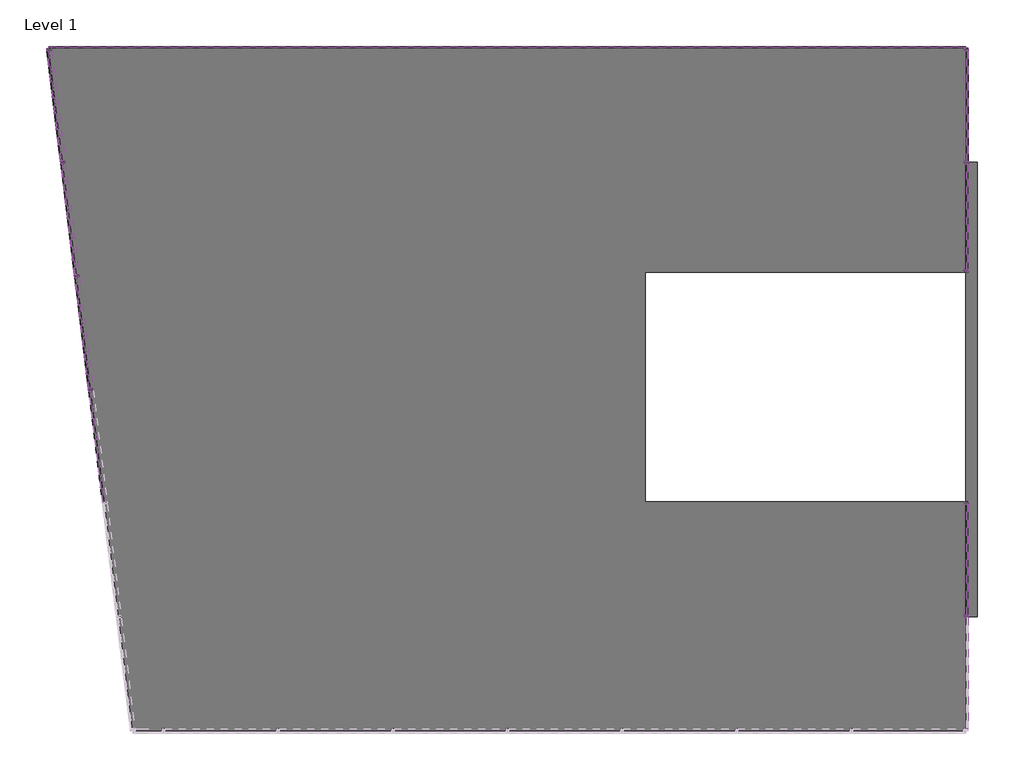
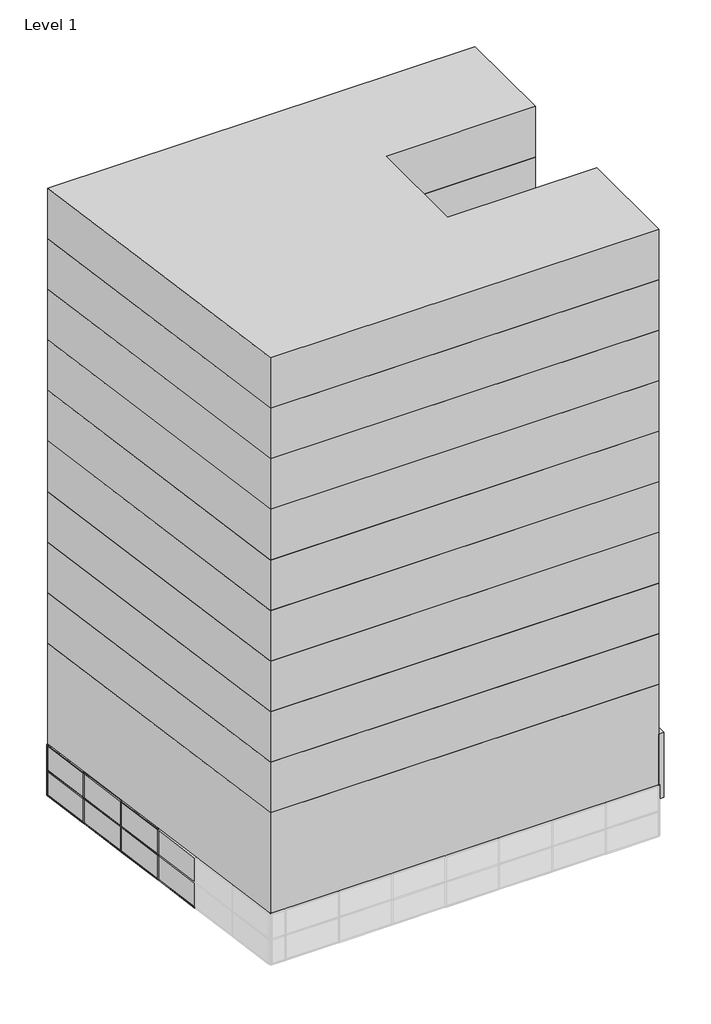
# One storey, part 2 of 2: 38 members, 30 plates, 2 proxies.
"""IFC4 building model written with IfcOpenShell, lengths in millimetres."""

from ifc_helpers import new_model, si_unit, frame, origin, origin_with_axes, place, context, project, spatial, polyline, outline, extrude, transform, mapped, element, save
from components import generic_models_1_generic_models_1_98a022ed, member_71c27fd2, member_19d0a4ec, member_8cef0660, member_db480205, member_82905deb, member_4491d118, member_1b94d493, member_46bdb8c2, system_panel_glazed_1e57f9bb, system_panel_glazed_37f15d2e, system_panel_glazed_3620f98e, system_panel_glazed_e46d4b42, system_panel_glazed_2a6c68b7, system_panel_glazed_7fb1fc2b, system_panel_glazed_d483336f

model = new_model("IFC4")

# Units and contexts
model_context = context("Model", 3, world=origin())
ifc_project = project(units=[si_unit("LENGTHUNIT", "METRE", prefix="MILLI")], contexts=[model_context])

# Site, building, storey
site = spatial("IfcSite", under=ifc_project)
building = spatial("IfcBuilding", under=site)
storey = spatial("IfcBuildingStorey", under=building, Name="Level 1", Elevation=0.0)

# Proxies
placement = place(None, origin())
generic_models_1_generic_models_1_shape = generic_models_1_generic_models_1_98a022ed(model_context)
element("IfcBuildingElementProxy", 1, Name="Generic Models 1 : Generic Models 1", ObjectType="Generic Models 1 : Generic Models 1", at=placement, inside=storey, context=model_context, shape_type="MappedRepresentation", body=[
    mapped(generic_models_1_generic_models_1_shape, transform((0.0, 0.0, 0.0), x_axis=(1.0, 0.0, 0.0), y_axis=(0.0, 1.0, 0.0), z_axis=(0.0, 0.0, 1.0))),
])
element("IfcBuildingElementProxy", 2, Name="Mass 1 : Mass 1", ObjectType="Mass 1 : Mass 1", at=placement, inside=storey, context=model_context, shape_type="SweptSolid", body=[
    extrude(outline(polyline([(13902.5156363, 11172.5476508), (13902.5156363, 5212.8636295), (5368.1156363, 5212.8636295), (5368.1156363, -883.1363705), (13902.5156363, -883.1363705), (13902.5156363, -6979.1363705), (-8252.7378115, -6979.1363705), (-10481.4843637, 11172.5476508), (13902.5156363, 11172.5476508)])), origin_with_axes(), (0.0, 0.0, 1.0), 9144.0),
    extrude(outline(polyline([(13902.5156363, 11172.5476508), (13902.5156363, 5212.8636295), (5368.1156363, 5212.8636295), (5368.1156363, -883.1363705), (13902.5156363, -883.1363705), (13902.5156363, -6979.1363705), (-8252.7378115, -6979.1363705), (-10481.4843637, 11172.5476508), (13902.5156363, 11172.5476508)])), origin_with_axes(), (0.0, 0.0, 1.0), 9144.0),
    extrude(outline(polyline([(13902.5156363, 11172.5476508), (13902.5156363, 5212.8636295), (5368.1156363, 5212.8636295), (5368.1156363, -883.1363705), (13902.5156363, -883.1363705), (13902.5156363, -6979.1363705), (-8252.7378115, -6979.1363705), (-10481.4843637, 11172.5476508), (13902.5156363, 11172.5476508)])), frame((0.0, 0.0, 3048.0), z_axis=(0.0, 0.0, 1.0), x_axis=(1.0, 0.0, 0.0)), (0.0, 0.0, 1.0), 9144.0),
    extrude(outline(polyline([(13902.5156363, 11172.5476508), (13902.5156363, 5212.8636295), (5368.1156363, 5212.8636295), (5368.1156363, -883.1363705), (13902.5156363, -883.1363705), (13902.5156363, -6979.1363705), (-8252.7378115, -6979.1363705), (-10481.4843637, 11172.5476508), (13902.5156363, 11172.5476508)])), frame((0.0, 0.0, 6096.0), z_axis=(0.0, 0.0, 1.0), x_axis=(1.0, 0.0, 0.0)), (0.0, 0.0, 1.0), 9144.0),
    extrude(outline(polyline([(13902.5156363, 11172.5476508), (13902.5156363, 5212.8636295), (5368.1156363, 5212.8636295), (5368.1156363, -883.1363705), (13902.5156363, -883.1363705), (13902.5156363, -6979.1363705), (-8252.7378115, -6979.1363705), (-10481.4843637, 11172.5476508), (13902.5156363, 11172.5476508)])), frame((0.0, 0.0, 9144.0), z_axis=(0.0, 0.0, 1.0), x_axis=(1.0, 0.0, 0.0)), (0.0, 0.0, 1.0), 9144.0),
    extrude(outline(polyline([(13902.5156363, 11172.5476508), (13902.5156363, 5212.8636295), (5368.1156363, 5212.8636295), (5368.1156363, -883.1363705), (13902.5156363, -883.1363705), (13902.5156363, -6979.1363705), (-8252.7378115, -6979.1363705), (-10481.4843637, 11172.5476508), (13902.5156363, 11172.5476508)])), frame((0.0, 0.0, 12192.0), z_axis=(0.0, 0.0, 1.0), x_axis=(1.0, 0.0, 0.0)), (0.0, 0.0, 1.0), 9144.0),
    extrude(outline(polyline([(13902.5156363, 11172.5476508), (13902.5156363, 5212.8636295), (5368.1156363, 5212.8636295), (5368.1156363, -883.1363705), (13902.5156363, -883.1363705), (13902.5156363, -6979.1363705), (-8252.7378115, -6979.1363705), (-10481.4843637, 11172.5476508), (13902.5156363, 11172.5476508)])), frame((0.0, 0.0, 15240.0), z_axis=(0.0, 0.0, 1.0), x_axis=(1.0, 0.0, 0.0)), (0.0, 0.0, 1.0), 9144.0),
    extrude(outline(polyline([(13902.5156363, 11172.5476508), (13902.5156363, 5212.8636295), (5368.1156363, 5212.8636295), (5368.1156363, -883.1363705), (13902.5156363, -883.1363705), (13902.5156363, -6979.1363705), (-8252.7378115, -6979.1363705), (-10481.4843637, 11172.5476508), (13902.5156363, 11172.5476508)])), frame((0.0, 0.0, 18288.0), z_axis=(0.0, 0.0, 1.0), x_axis=(1.0, 0.0, 0.0)), (0.0, 0.0, 1.0), 9144.0),
    extrude(outline(polyline([(13902.5156363, 11172.5476508), (13902.5156363, 5212.8636295), (5368.1156363, 5212.8636295), (5368.1156363, -883.1363705), (13902.5156363, -883.1363705), (13902.5156363, -6979.1363705), (-8252.7378115, -6979.1363705), (-10481.4843637, 11172.5476508), (13902.5156363, 11172.5476508)])), frame((0.0, 0.0, 21336.0), z_axis=(0.0, 0.0, 1.0), x_axis=(1.0, 0.0, 0.0)), (0.0, 0.0, 1.0), 9144.0),
    extrude(outline(polyline([(13902.5156363, 11172.5476508), (13902.5156363, 5212.8636295), (5368.1156363, 5212.8636295), (5368.1156363, -883.1363705), (13902.5156363, -883.1363705), (13902.5156363, -6979.1363705), (-8252.7378115, -6979.1363705), (-10481.4843637, 11172.5476508), (13902.5156363, 11172.5476508)])), frame((0.0, 0.0, 24384.0), z_axis=(0.0, 0.0, 1.0), x_axis=(1.0, 0.0, 0.0)), (0.0, 0.0, 1.0), 9144.0),
    extrude(outline(polyline([(13902.5156363, 11172.5476508), (13902.5156363, 5212.8636295), (5368.1156363, 5212.8636295), (5368.1156363, -883.1363705), (13902.5156363, -883.1363705), (13902.5156363, -6979.1363705), (-8252.7378115, -6979.1363705), (-10481.4843637, 11172.5476508), (13902.5156363, 11172.5476508)])), frame((0.0, 0.0, 27432.0), z_axis=(0.0, 0.0, 1.0), x_axis=(1.0, 0.0, 0.0)), (0.0, 0.0, 1.0), 9144.0),
])

# Members
member_shape = member_71c27fd2(model_context)
element("IfcMember", 3, ObjectType="Rectangular Mullion : 2.5\" x 5\" rectangular", at=placement, inside=storey, context=model_context, shape_type="MappedRepresentation", body=[
    mapped(member_shape, transform((-10473.7456604, 11109.5209701, 0.0), x_axis=(0.0, 0.0, -1.0), y_axis=(-0.9925461516413222, -0.12186934340514595, 0.0), z_axis=(-0.12186934340514594, 0.9925461516413221, 0.0))),
])
element("IfcMember", 4, ObjectType="Rectangular Mullion : 2.5\" x 5\" rectangular", at=placement, inside=storey, context=model_context, shape_type="MappedRepresentation", body=[
    mapped(member_shape, transform((13902.5156363, 8156.2976505, 0.0), x_axis=(0.0, 0.0, -1.0), y_axis=(1.0, 0.0, 0.0), z_axis=(0.0, -1.0, 0.0))),
])
element("IfcMember", 5, ObjectType="Rectangular Mullion : 2.5\" x 5\" rectangular", at=placement, inside=storey, context=model_context, shape_type="MappedRepresentation", body=[
    mapped(member_shape, transform((13902.5156363, -3899.3863708, 0.0), x_axis=(0.0, 0.0, -1.0), y_axis=(1.0, 0.0, 0.0), z_axis=(0.0, -1.0, 0.0))),
])
member_2_shape = member_19d0a4ec(model_context)
element("IfcMember", 6, ObjectType="Rectangular Mullion : 2.5\" x 5\" rectangular", at=placement, inside=storey, context=model_context, shape_type="MappedRepresentation", body=[
    mapped(member_2_shape, transform((-10113.8959567, 8178.7803212, 1524.0), x_axis=(0.0, 0.0, 1.0), y_axis=(-0.9925461516413222, -0.12186934340514595, 0.0), z_axis=(0.12186934340514594, -0.9925461516413221, 0.0))),
])
element("IfcMember", 7, ObjectType="Rectangular Mullion : 2.5\" x 5\" rectangular", at=placement, inside=storey, context=model_context, shape_type="MappedRepresentation", body=[
    mapped(member_2_shape, transform((-10113.8959567, 8178.7803212, 3048.0), x_axis=(0.0, 0.0, 1.0), y_axis=(-0.9925461516413222, -0.12186934340514595, 0.0), z_axis=(0.12186934340514594, -0.9925461516413221, 0.0))),
])
element("IfcMember", 8, ObjectType="Rectangular Mullion : 2.5\" x 5\" rectangular", at=placement, inside=storey, context=model_context, shape_type="MappedRepresentation", body=[
    mapped(member_2_shape, transform((13902.5156363, 11109.0476508, 1524.0), x_axis=(0.0, 0.0, 1.0), y_axis=(1.0, 0.0, 0.0), z_axis=(0.0, 1.0, 0.0))),
])
element("IfcMember", 9, ObjectType="Rectangular Mullion : 2.5\" x 5\" rectangular", at=placement, inside=storey, context=model_context, shape_type="MappedRepresentation", body=[
    mapped(member_2_shape, transform((13902.5156363, 11109.0476508, 3048.0), x_axis=(0.0, 0.0, 1.0), y_axis=(1.0, 0.0, 0.0), z_axis=(0.0, 1.0, 0.0))),
])
element("IfcMember", 10, ObjectType="Rectangular Mullion : 2.5\" x 5\" rectangular", at=placement, inside=storey, context=model_context, shape_type="MappedRepresentation", body=[
    mapped(member_2_shape, transform((13902.5156363, -946.6363705, 1524.0), x_axis=(0.0, 0.0, 1.0), y_axis=(1.0, 0.0, 0.0), z_axis=(0.0, 1.0, 0.0))),
])
element("IfcMember", 11, ObjectType="Rectangular Mullion : 2.5\" x 5\" rectangular", at=placement, inside=storey, context=model_context, shape_type="MappedRepresentation", body=[
    mapped(member_2_shape, transform((13902.5156363, -946.6363705, 3048.0), x_axis=(0.0, 0.0, 1.0), y_axis=(1.0, 0.0, 0.0), z_axis=(0.0, 1.0, 0.0))),
])
element("IfcMember", 12, ObjectType="Rectangular Mullion : 2.5\" x 5\" rectangular", at=placement, inside=storey, context=model_context, shape_type="MappedRepresentation", body=[
    mapped(member_2_shape, transform((13902.5156363, -3962.8863708, 3048.0), x_axis=(0.0, 0.0, 1.0), y_axis=(1.0, 0.0, 0.0), z_axis=(0.0, 1.0, 0.0))),
])
member_3_shape = member_8cef0660(model_context)
element("IfcMember", 13, ObjectType="Rectangular Mullion : 2.5\" x 5\" rectangular", at=placement, inside=storey, context=model_context, shape_type="MappedRepresentation", body=[
    mapped(member_3_shape, transform((-9370.9804393, 2128.2189808, 1524.0), x_axis=(0.0, 0.0, 1.0), y_axis=(-0.9925461516413222, -0.12186934340514596, 0.0), z_axis=(0.12186934340514596, -0.9925461516413222, 0.0))),
])
element("IfcMember", 14, ObjectType="Rectangular Mullion : 2.5\" x 5\" rectangular", at=placement, inside=storey, context=model_context, shape_type="MappedRepresentation", body=[
    mapped(member_3_shape, transform((-9742.438198, 5153.499651, 1524.0), x_axis=(0.0, 0.0, 1.0), y_axis=(-0.9925461516413222, -0.12186934340514596, 0.0), z_axis=(0.12186934340514596, -0.9925461516413222, 0.0))),
])
element("IfcMember", 15, ObjectType="Rectangular Mullion : 2.5\" x 5\" rectangular", at=placement, inside=storey, context=model_context, shape_type="MappedRepresentation", body=[
    mapped(member_3_shape, transform((-9370.9804393, 2128.2189808, 3048.0), x_axis=(0.0, 0.0, 1.0), y_axis=(-0.9925461516413223, -0.12186934340514563, 0.0), z_axis=(0.12186934340514562, -0.9925461516413222, 0.0))),
])
element("IfcMember", 16, ObjectType="Rectangular Mullion : 2.5\" x 5\" rectangular", at=placement, inside=storey, context=model_context, shape_type="MappedRepresentation", body=[
    mapped(member_3_shape, transform((-9742.438198, 5153.499651, 3048.0), x_axis=(0.0, 0.0, 1.0), y_axis=(-0.9925461516413222, -0.12186934340514596, 0.0), z_axis=(0.12186934340514596, -0.9925461516413222, 0.0))),
])
member_4_shape = member_db480205(model_context)
element("IfcMember", 17, ObjectType="Rectangular Mullion : 2.5\" x 5\" rectangular", at=placement, inside=storey, context=model_context, shape_type="MappedRepresentation", body=[
    mapped(member_4_shape, transform((-9363.241736, 2065.1923001, 0.0), x_axis=(0.0, 0.0, -1.0), y_axis=(-0.9925461516413222, -0.12186934340514566, 0.0), z_axis=(-0.12186934340514566, 0.9925461516413222, 0.0))),
])
element("IfcMember", 18, ObjectType="Rectangular Mullion : 2.5\" x 5\" rectangular", at=placement, inside=storey, context=model_context, shape_type="MappedRepresentation", body=[
    mapped(member_4_shape, transform((-9734.6994947, 5090.4729703, 0.0), x_axis=(0.0, 0.0, -1.0), y_axis=(-0.9925461516413222, -0.12186934340514596, 0.0), z_axis=(-0.12186934340514596, 0.9925461516413222, 0.0))),
])
element("IfcMember", 19, ObjectType="Rectangular Mullion : 2.5\" x 5\" rectangular", at=placement, inside=storey, context=model_context, shape_type="MappedRepresentation", body=[
    mapped(member_4_shape, transform((-10106.1572534, 8115.7536405, 0.0), x_axis=(0.0, 0.0, -1.0), y_axis=(-0.9925461516413222, -0.12186934340514596, 0.0), z_axis=(-0.12186934340514596, 0.9925461516413222, 0.0))),
])
member_5_shape = member_82905deb(model_context)
element("IfcMember", 20, ObjectType="Rectangular Mullion : 2.5\" x 5\" rectangular", at=placement, inside=storey, context=model_context, shape_type="MappedRepresentation", body=[
    mapped(member_5_shape, transform((-9367.1110876, 2096.7056405, 1524.0), x_axis=(-0.12186934340514591, 0.9925461516413222, 0.0), y_axis=(-0.9925461516413222, -0.12186934340514591, 0.0), z_axis=(0.0, 0.0, 1.0))),
])
element("IfcMember", 21, ObjectType="Rectangular Mullion : 2.5\" x 5\" rectangular", at=placement, inside=storey, context=model_context, shape_type="MappedRepresentation", body=[
    mapped(member_5_shape, transform((-9738.5688463, 5121.9863107, 1524.0), x_axis=(-0.12186934340514591, 0.9925461516413222, 0.0), y_axis=(-0.9925461516413222, -0.12186934340514591, 0.0), z_axis=(0.0, 0.0, 1.0))),
])
element("IfcMember", 22, ObjectType="Rectangular Mullion : 2.5\" x 5\" rectangular", at=placement, inside=storey, context=model_context, shape_type="MappedRepresentation", body=[
    mapped(member_5_shape, transform((-10110.026605, 8147.2669809, 1524.0), x_axis=(-0.12186934340514591, 0.9925461516413222, 0.0), y_axis=(-0.9925461516413222, -0.12186934340514591, 0.0), z_axis=(0.0, 0.0, 1.0))),
])
element("IfcMember", 23, ObjectType="Rectangular Mullion : 2.5\" x 5\" rectangular", at=placement, inside=storey, context=model_context, shape_type="MappedRepresentation", body=[
    mapped(member_5_shape, transform((13902.5156363, 8124.5476505, 1524.0), x_axis=(0.0, -1.0, 0.0), y_axis=(1.0, 0.0, 0.0), z_axis=(0.0, 0.0, 1.0))),
])
element("IfcMember", 24, ObjectType="Rectangular Mullion : 2.5\" x 5\" rectangular", at=placement, inside=storey, context=model_context, shape_type="MappedRepresentation", body=[
    mapped(member_5_shape, transform((13902.5156363, -3931.1363708, 1524.0), x_axis=(0.0, -1.0, 0.0), y_axis=(1.0, 0.0, 0.0), z_axis=(0.0, 0.0, 1.0))),
])
element("IfcMember", 25, ObjectType="Rectangular Mullion : 2.5\" x 5\" rectangular", at=placement, inside=storey, context=model_context, shape_type="MappedRepresentation", body=[
    mapped(member_5_shape, transform((-9367.1110876, 2096.7056405, 3048.0), x_axis=(-0.12186934340514591, 0.9925461516413222, 0.0), y_axis=(-0.9925461516413222, -0.12186934340514591, 0.0), z_axis=(0.0, 0.0, 1.0))),
])
element("IfcMember", 26, ObjectType="Rectangular Mullion : 2.5\" x 5\" rectangular", at=placement, inside=storey, context=model_context, shape_type="MappedRepresentation", body=[
    mapped(member_5_shape, transform((-9738.5688463, 5121.9863107, 3048.0), x_axis=(-0.12186934340514591, 0.9925461516413222, 0.0), y_axis=(-0.9925461516413222, -0.12186934340514591, 0.0), z_axis=(0.0, 0.0, 1.0))),
])
element("IfcMember", 27, ObjectType="Rectangular Mullion : 2.5\" x 5\" rectangular", at=placement, inside=storey, context=model_context, shape_type="MappedRepresentation", body=[
    mapped(member_5_shape, transform((-10110.026605, 8147.2669809, 3048.0), x_axis=(-0.12186934340514591, 0.9925461516413222, 0.0), y_axis=(-0.9925461516413222, -0.12186934340514591, 0.0), z_axis=(0.0, 0.0, 1.0))),
])
element("IfcMember", 28, ObjectType="Rectangular Mullion : 2.5\" x 5\" rectangular", at=placement, inside=storey, context=model_context, shape_type="MappedRepresentation", body=[
    mapped(member_5_shape, transform((13902.5156363, 8124.5476505, 3048.0), x_axis=(0.0, -1.0, 0.0), y_axis=(1.0, 0.0, 0.0), z_axis=(0.0, 0.0, 1.0))),
])
element("IfcMember", 29, ObjectType="Rectangular Mullion : 2.5\" x 5\" rectangular", at=placement, inside=storey, context=model_context, shape_type="MappedRepresentation", body=[
    mapped(member_5_shape, transform((13902.5156363, -3931.1363708, 3048.0), x_axis=(0.0, -1.0, 0.0), y_axis=(1.0, 0.0, 0.0), z_axis=(0.0, 0.0, 1.0))),
])
member_6_shape = member_4491d118(model_context)
element("IfcMember", 30, ObjectType="Rectangular Mullion : 2.5\" x 5\" rectangular", at=placement, inside=storey, context=model_context, shape_type="MappedRepresentation", body=[
    mapped(member_6_shape, transform((13902.5156363, 11172.5476508, 0.0), x_axis=(0.0, 1.0, 0.0), y_axis=(1.0, 0.0, 0.0), z_axis=(0.0, 0.0, -1.0))),
])
element("IfcMember", 31, ObjectType="Rectangular Mullion : 2.5\" x 5\" rectangular", at=placement, inside=storey, context=model_context, shape_type="MappedRepresentation", body=[
    mapped(member_6_shape, transform((13902.5156363, -883.1363705, 0.0), x_axis=(0.0, 1.0, 0.0), y_axis=(1.0, 0.0, 0.0), z_axis=(0.0, 0.0, -1.0))),
])
element("IfcMember", 32, ObjectType="Rectangular Mullion : 2.5\" x 5\" rectangular", at=placement, inside=storey, context=model_context, shape_type="MappedRepresentation", body=[
    mapped(member_6_shape, transform((13902.5156363, 11172.5476508, 1524.0), x_axis=(0.0, 1.0, 0.0), y_axis=(1.0, 0.0, 0.0), z_axis=(0.0, 0.0, -1.0))),
])
element("IfcMember", 33, ObjectType="Rectangular Mullion : 2.5\" x 5\" rectangular", at=placement, inside=storey, context=model_context, shape_type="MappedRepresentation", body=[
    mapped(member_6_shape, transform((13902.5156363, -883.1363705, 1524.0), x_axis=(0.0, 1.0, 0.0), y_axis=(1.0, 0.0, 0.0), z_axis=(0.0, 0.0, -1.0))),
])
element("IfcMember", 34, ObjectType="Rectangular Mullion : 2.5\" x 5\" rectangular", at=placement, inside=storey, context=model_context, shape_type="MappedRepresentation", body=[
    mapped(member_6_shape, transform((-10481.4843637, 11172.5476508, 1524.0), x_axis=(-0.12186934340514591, 0.9925461516413222, 0.0), y_axis=(-0.9925461516413222, -0.12186934340514591, 0.0), z_axis=(0.0, 0.0, 1.0))),
])
element("IfcMember", 35, ObjectType="Rectangular Mullion : 2.5\" x 5\" rectangular", at=placement, inside=storey, context=model_context, shape_type="MappedRepresentation", body=[
    mapped(member_6_shape, transform((13902.5156363, 5212.8636295, 1524.0), x_axis=(0.0, -1.0, 0.0), y_axis=(1.0, 0.0, 0.0), z_axis=(0.0, 0.0, 1.0))),
])
element("IfcMember", 36, ObjectType="Rectangular Mullion : 2.5\" x 5\" rectangular", at=placement, inside=storey, context=model_context, shape_type="MappedRepresentation", body=[
    mapped(member_6_shape, transform((-10481.4843637, 11172.5476508, 3048.0), x_axis=(-0.12186934340514591, 0.9925461516413222, 0.0), y_axis=(-0.9925461516413222, -0.12186934340514591, 0.0), z_axis=(0.0, 0.0, 1.0))),
])
element("IfcMember", 37, ObjectType="Rectangular Mullion : 2.5\" x 5\" rectangular", at=placement, inside=storey, context=model_context, shape_type="MappedRepresentation", body=[
    mapped(member_6_shape, transform((13902.5156363, 5212.8636295, 3048.0), x_axis=(0.0, -1.0, 0.0), y_axis=(1.0, 0.0, 0.0), z_axis=(0.0, 0.0, 1.0))),
])
member_7_shape = member_1b94d493(model_context)
element("IfcMember", 38, ObjectType="Rectangular Mullion : 2.5\" x 5\" rectangular", at=placement, inside=storey, context=model_context, shape_type="MappedRepresentation", body=[
    mapped(member_7_shape, transform((13902.5156363, 5276.3636295, 0.0), x_axis=(0.0, 0.0, -1.0), y_axis=(1.0, 0.0, 0.0), z_axis=(0.0, -1.0, 0.0))),
])
member_8_shape = member_46bdb8c2(model_context)
element("IfcMember", 39, ObjectType="Rectangular Mullion : 2.5\" x 5\" rectangular", at=placement, inside=storey, context=model_context, shape_type="MappedRepresentation", body=[
    mapped(member_8_shape, transform((13902.5156363, 8092.7976505, 1524.0), x_axis=(0.0, 0.0, 1.0), y_axis=(1.0, 0.0, 0.0), z_axis=(0.0, 1.0, 0.0))),
])
element("IfcMember", 40, ObjectType="Rectangular Mullion : 2.5\" x 5\" rectangular", at=placement, inside=storey, context=model_context, shape_type="MappedRepresentation", body=[
    mapped(member_8_shape, transform((13902.5156363, 8092.7976505, 3048.0), x_axis=(0.0, 0.0, 1.0), y_axis=(1.0, 0.0, 0.0), z_axis=(0.0, 1.0, 0.0))),
])

# Plates
system_panel_glazed_shape = system_panel_glazed_1e57f9bb(model_context)
element("IfcPlate", 41, ObjectType="System Panel : Glazed", at=placement, inside=storey, context=model_context, shape_type="MappedRepresentation", body=[
    mapped(system_panel_glazed_shape, transform((-8957.4843636, 11172.5476508, 0.0), x_axis=(1.0, 0.0, 0.0), y_axis=(0.0, 1.0, 0.0), z_axis=(0.0, 0.0, 1.0))),
])
element("IfcPlate", 42, ObjectType="System Panel : Glazed", at=placement, inside=storey, context=model_context, shape_type="MappedRepresentation", body=[
    mapped(system_panel_glazed_shape, transform((-5909.4843634, 11172.5476508, 0.0), x_axis=(1.0, 0.0, 0.0), y_axis=(0.0, 1.0, 0.0), z_axis=(0.0, 0.0, 1.0))),
])
element("IfcPlate", 43, ObjectType="System Panel : Glazed", at=placement, inside=storey, context=model_context, shape_type="MappedRepresentation", body=[
    mapped(system_panel_glazed_shape, transform((-2861.4843634, 11172.5476508, 0.0), x_axis=(1.0, 0.0, 0.0), y_axis=(0.0, 1.0, 0.0), z_axis=(0.0, 0.0, 1.0))),
])
element("IfcPlate", 44, ObjectType="System Panel : Glazed", at=placement, inside=storey, context=model_context, shape_type="MappedRepresentation", body=[
    mapped(system_panel_glazed_shape, transform((186.5156366, 11172.5476508, 0.0), x_axis=(1.0, 0.0, 0.0), y_axis=(0.0, 1.0, 0.0), z_axis=(0.0, 0.0, 1.0))),
])
element("IfcPlate", 45, ObjectType="System Panel : Glazed", at=placement, inside=storey, context=model_context, shape_type="MappedRepresentation", body=[
    mapped(system_panel_glazed_shape, transform((3234.5156366, 11172.5476508, 0.0), x_axis=(1.0, 0.0, 0.0), y_axis=(0.0, 1.0, 0.0), z_axis=(0.0, 0.0, 1.0))),
])
element("IfcPlate", 46, ObjectType="System Panel : Glazed", at=placement, inside=storey, context=model_context, shape_type="MappedRepresentation", body=[
    mapped(system_panel_glazed_shape, transform((6282.5156366, 11172.5476508, 0.0), x_axis=(1.0, 0.0, 0.0), y_axis=(0.0, 1.0, 0.0), z_axis=(0.0, 0.0, 1.0))),
])
element("IfcPlate", 47, ObjectType="System Panel : Glazed", at=placement, inside=storey, context=model_context, shape_type="MappedRepresentation", body=[
    mapped(system_panel_glazed_shape, transform((9330.5156366, 11172.5476508, 0.0), x_axis=(1.0, 0.0, 0.0), y_axis=(0.0, 1.0, 0.0), z_axis=(0.0, 0.0, 1.0))),
])
element("IfcPlate", 48, ObjectType="System Panel : Glazed", at=placement, inside=storey, context=model_context, shape_type="MappedRepresentation", body=[
    mapped(system_panel_glazed_shape, transform((12378.5156364, 11172.5476508, 0.0), x_axis=(1.0, 0.0, 0.0), y_axis=(0.0, 1.0, 0.0), z_axis=(0.0, 0.0, 1.0))),
])
element("IfcPlate", 49, ObjectType="System Panel : Glazed", at=placement, inside=storey, context=model_context, shape_type="MappedRepresentation", body=[
    mapped(system_panel_glazed_shape, transform((-8957.4843636, 11172.5476508, 1524.0), x_axis=(1.0, 0.0, 0.0), y_axis=(0.0, 1.0, 0.0), z_axis=(0.0, 0.0, 1.0))),
])
element("IfcPlate", 50, ObjectType="System Panel : Glazed", at=placement, inside=storey, context=model_context, shape_type="MappedRepresentation", body=[
    mapped(system_panel_glazed_shape, transform((-5909.4843634, 11172.5476508, 1524.0), x_axis=(1.0, 0.0, 0.0), y_axis=(0.0, 1.0, 0.0), z_axis=(0.0, 0.0, 1.0))),
])
element("IfcPlate", 51, ObjectType="System Panel : Glazed", at=placement, inside=storey, context=model_context, shape_type="MappedRepresentation", body=[
    mapped(system_panel_glazed_shape, transform((-2861.4843634, 11172.5476508, 1524.0), x_axis=(1.0, 0.0, 0.0), y_axis=(0.0, 1.0, 0.0), z_axis=(0.0, 0.0, 1.0))),
])
element("IfcPlate", 52, ObjectType="System Panel : Glazed", at=placement, inside=storey, context=model_context, shape_type="MappedRepresentation", body=[
    mapped(system_panel_glazed_shape, transform((186.5156366, 11172.5476508, 1524.0), x_axis=(1.0, 0.0, 0.0), y_axis=(0.0, 1.0, 0.0), z_axis=(0.0, 0.0, 1.0))),
])
element("IfcPlate", 53, ObjectType="System Panel : Glazed", at=placement, inside=storey, context=model_context, shape_type="MappedRepresentation", body=[
    mapped(system_panel_glazed_shape, transform((3234.5156366, 11172.5476508, 1524.0), x_axis=(1.0, 0.0, 0.0), y_axis=(0.0, 1.0, 0.0), z_axis=(0.0, 0.0, 1.0))),
])
element("IfcPlate", 54, ObjectType="System Panel : Glazed", at=placement, inside=storey, context=model_context, shape_type="MappedRepresentation", body=[
    mapped(system_panel_glazed_shape, transform((6282.5156366, 11172.5476508, 1524.0), x_axis=(1.0, 0.0, 0.0), y_axis=(0.0, 1.0, 0.0), z_axis=(0.0, 0.0, 1.0))),
])
element("IfcPlate", 55, ObjectType="System Panel : Glazed", at=placement, inside=storey, context=model_context, shape_type="MappedRepresentation", body=[
    mapped(system_panel_glazed_shape, transform((9330.5156366, 11172.5476508, 1524.0), x_axis=(1.0, 0.0, 0.0), y_axis=(0.0, 1.0, 0.0), z_axis=(0.0, 0.0, 1.0))),
])
element("IfcPlate", 56, ObjectType="System Panel : Glazed", at=placement, inside=storey, context=model_context, shape_type="MappedRepresentation", body=[
    mapped(system_panel_glazed_shape, transform((12378.5156364, 11172.5476508, 1524.0), x_axis=(1.0, 0.0, 0.0), y_axis=(0.0, 1.0, 0.0), z_axis=(0.0, 0.0, 1.0))),
])
system_panel_glazed_2_shape = system_panel_glazed_37f15d2e(model_context)
element("IfcPlate", 57, ObjectType="System Panel : Glazed", at=placement, inside=storey, context=model_context, shape_type="MappedRepresentation", body=[
    mapped(system_panel_glazed_2_shape, transform((13902.5156363, -2423.0113706, 63.5), x_axis=(0.0, -1.0, 0.0), y_axis=(1.0, 0.0, 0.0), z_axis=(0.0, 0.0, 1.0))),
])
element("IfcPlate", 58, ObjectType="System Panel : Glazed", at=placement, inside=storey, context=model_context, shape_type="MappedRepresentation", body=[
    mapped(system_panel_glazed_2_shape, transform((13902.5156363, 9632.6726506, 63.5), x_axis=(0.0, -1.0, 0.0), y_axis=(1.0, 0.0, 0.0), z_axis=(0.0, 0.0, 1.0))),
])
element("IfcPlate", 59, ObjectType="System Panel : Glazed", at=placement, inside=storey, context=model_context, shape_type="MappedRepresentation", body=[
    mapped(system_panel_glazed_2_shape, transform((-10293.8208085, 9644.1506457, 63.5), x_axis=(-0.12186934340514591, 0.9925461516413222, 0.0), y_axis=(-0.9925461516413222, -0.12186934340514591, 0.0), z_axis=(0.0, 0.0, 1.0))),
])
system_panel_glazed_3_shape = system_panel_glazed_3620f98e(model_context)
element("IfcPlate", 60, ObjectType="System Panel : Glazed", at=placement, inside=storey, context=model_context, shape_type="MappedRepresentation", body=[
    mapped(system_panel_glazed_3_shape, transform((-9181.3822083, 584.0653054, 63.5), x_axis=(-0.12186934340514591, 0.9925461516413222, 0.0), y_axis=(-0.9925461516413222, -0.12186934340514591, 0.0), z_axis=(0.0, 0.0, 1.0))),
])
element("IfcPlate", 61, ObjectType="System Panel : Glazed", at=placement, inside=storey, context=model_context, shape_type="MappedRepresentation", body=[
    mapped(system_panel_glazed_3_shape, transform((-9552.839967, 3609.3459756, 63.5), x_axis=(-0.12186934340514591, 0.9925461516413222, 0.0), y_axis=(-0.9925461516413222, -0.12186934340514591, 0.0), z_axis=(0.0, 0.0, 1.0))),
])
element("IfcPlate", 62, ObjectType="System Panel : Glazed", at=placement, inside=storey, context=model_context, shape_type="MappedRepresentation", body=[
    mapped(system_panel_glazed_3_shape, transform((-9924.2977257, 6634.6266458, 63.5), x_axis=(-0.12186934340514591, 0.9925461516413222, 0.0), y_axis=(-0.9925461516413222, -0.12186934340514591, 0.0), z_axis=(0.0, 0.0, 1.0))),
])
system_panel_glazed_4_shape = system_panel_glazed_e46d4b42(model_context)
element("IfcPlate", 63, ObjectType="System Panel : Glazed", at=placement, inside=storey, context=model_context, shape_type="MappedRepresentation", body=[
    mapped(system_panel_glazed_4_shape, transform((-10293.8208085, 9644.1506457, 1555.75), x_axis=(-0.12186934340514591, 0.9925461516413222, 0.0), y_axis=(-0.9925461516413222, -0.12186934340514591, 0.0), z_axis=(0.0, 0.0, 1.0))),
])
element("IfcPlate", 64, ObjectType="System Panel : Glazed", at=placement, inside=storey, context=model_context, shape_type="MappedRepresentation", body=[
    mapped(system_panel_glazed_4_shape, transform((13902.5156363, -2423.0113706, 1555.75), x_axis=(0.0, -1.0, 0.0), y_axis=(1.0, 0.0, 0.0), z_axis=(0.0, 0.0, 1.0))),
])
element("IfcPlate", 65, ObjectType="System Panel : Glazed", at=placement, inside=storey, context=model_context, shape_type="MappedRepresentation", body=[
    mapped(system_panel_glazed_4_shape, transform((13902.5156363, 9632.6726506, 1555.75), x_axis=(0.0, -1.0, 0.0), y_axis=(1.0, 0.0, 0.0), z_axis=(0.0, 0.0, 1.0))),
])
system_panel_glazed_5_shape = system_panel_glazed_2a6c68b7(model_context)
element("IfcPlate", 66, ObjectType="System Panel : Glazed", at=placement, inside=storey, context=model_context, shape_type="MappedRepresentation", body=[
    mapped(system_panel_glazed_5_shape, transform((-9181.3822083, 584.0653054, 1555.75), x_axis=(-0.12186934340514591, 0.9925461516413222, 0.0), y_axis=(-0.9925461516413222, -0.12186934340514591, 0.0), z_axis=(0.0, 0.0, 1.0))),
])
element("IfcPlate", 67, ObjectType="System Panel : Glazed", at=placement, inside=storey, context=model_context, shape_type="MappedRepresentation", body=[
    mapped(system_panel_glazed_5_shape, transform((-9552.839967, 3609.3459756, 1555.75), x_axis=(-0.12186934340514591, 0.9925461516413222, 0.0), y_axis=(-0.9925461516413222, -0.12186934340514591, 0.0), z_axis=(0.0, 0.0, 1.0))),
])
element("IfcPlate", 68, ObjectType="System Panel : Glazed", at=placement, inside=storey, context=model_context, shape_type="MappedRepresentation", body=[
    mapped(system_panel_glazed_5_shape, transform((-9924.2977257, 6634.6266458, 1555.75), x_axis=(-0.12186934340514591, 0.9925461516413222, 0.0), y_axis=(-0.9925461516413222, -0.12186934340514591, 0.0), z_axis=(0.0, 0.0, 1.0))),
])
system_panel_glazed_6_shape = system_panel_glazed_7fb1fc2b(model_context)
element("IfcPlate", 69, ObjectType="System Panel : Glazed", at=placement, inside=storey, context=model_context, shape_type="MappedRepresentation", body=[
    mapped(system_panel_glazed_6_shape, transform((13902.5156363, 6684.58064, 63.5), x_axis=(0.0, -1.0, 0.0), y_axis=(1.0, 0.0, 0.0), z_axis=(0.0, 0.0, 1.0))),
])
system_panel_glazed_7_shape = system_panel_glazed_d483336f(model_context)
element("IfcPlate", 70, ObjectType="System Panel : Glazed", at=placement, inside=storey, context=model_context, shape_type="MappedRepresentation", body=[
    mapped(system_panel_glazed_7_shape, transform((13902.5156363, 6684.58064, 1555.75), x_axis=(0.0, -1.0, 0.0), y_axis=(1.0, 0.0, 0.0), z_axis=(0.0, 0.0, 1.0))),
])

save(model, "model.ifc")

# Revit data of these elements
# Type "Rectangular Mullion : 2.5\" x 5\" rectangular"
#   built-in parameter 1007304 = 0.416667 (stored number, unit not read)
#   built-in parameter 1007301 = 0.104167 (stored number, unit not read)
#   built-in parameter 1007300 = 0.104167 (stored number, unit not read)
# Type "System Panel : Glazed"
#   Construction Type Id = "GSP4R"
#   Analytic Construction = "1/8 in Pilkington single glazing"
#   Visual Light Transmittance = 0.9
#   Solar Heat Gain Coefficient = 0.86
#   Heat Transfer Coefficient (U) = 1.18115 BTU/(h·ft²·°F)
#   Define Thermal Properties by = 1
# Element 1 (IfcBuildingElementProxy, "Generic Models 1 : Generic Models 1")
#   Phase Created = New Construction
# Element 2 (IfcBuildingElementProxy, "Mass 1 : Mass 1")
#   Phase Created = New Construction
#   Materials on its faces: "Default Form"
# Elements 3, 4, 5, 6, 7, 8, 9, 10, 11, 12, 13, 14, 15, 16, 17, 18, 19, 20, 21, 22, 23, 24, 25, 26, 27, 28, 29, 30, 31, 32, 33, 34, 35, 36, 37, 38, 39, 40 (IfcMember, "Rectangular Mullion : 2.5\" x 5\" rectangular")
#   Phase Created = New Construction
#   Materials on its faces: "Aluminum"
# Elements 41, 42, 43, 44, 45, 46, 47, 48, 49, 50, 51, 52, 53, 54, 55, 56, 57, 58, 59, 60, 61, 62, 63, 64, 65, 66, 67, 68, 69, 70 (IfcPlate, "System Panel : Glazed")
#   Phase Created = New Construction
#   Materials on its faces: "Glass"
# Materials
#   "Default Form": class "Generic", colour RGB 185 189 196, transparency 0.5, Cost = 0
#   "Aluminum": class "Metal", colour RGB 247 247 247, transparency 0, Description = "Aluminum 6061", Cost = 0
#   "Glass": class "Glass", colour RGB 0 128 192, transparency 0.75, Description = "Soda Lime Glass", Cost = 0
